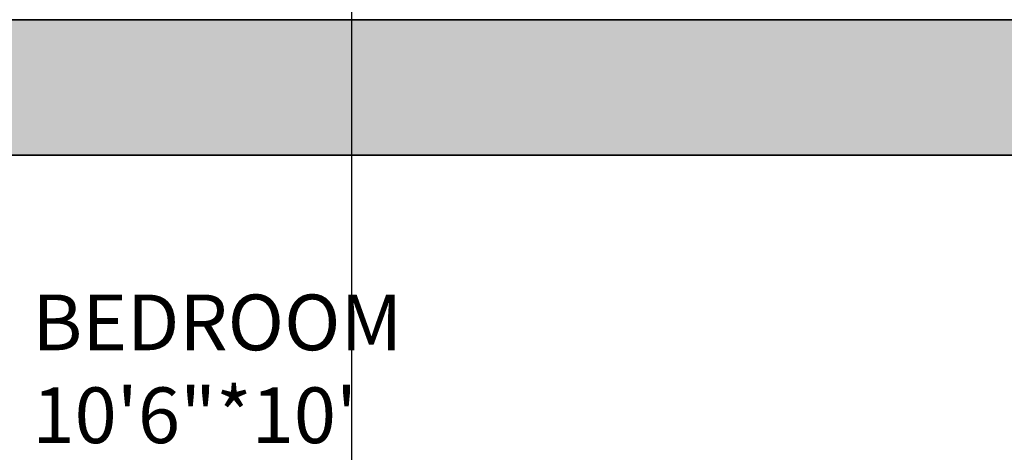
# Model space of a CAD drawing. Units: inches. Extents: x 1998 to 2588, y 1139 to 1977.
# Tile 74 of 134: x 2126 to 2192, y 1860 to 1889. Entities that reach past the tile are written whole.
import ezdxf

# ---------------------------------------------------------------- set-up
doc = ezdxf.new("R2010")
doc.units = ezdxf.units.IN
for name, color, linetype, lineweight in [('A-ANNO-DIMS', 2, 'Continuous', 18), ('A-AREA-IDEN', 7, 'Continuous', 18), ('A-WALL-PATT', 252, 'Continuous', 13), ('WALL', 200, 'Continuous', 35)]:
    doc.layers.add(name, color=color, linetype=linetype, lineweight=lineweight)
doc.styles.get("Standard").update_dxf_attribs({"font": 'arial.ttf'})
doc.dimstyles.get("Standard").update_dxf_attribs({"dimtxt": 0.18, "dimasz": 0.18, "dimexe": 0.18, "dimexo": 0.0625, "dimgap": 0.09, "dimtad": 0, "dimtih": 1, "dimtoh": 1, "dimdec": 4, "dimzin": 0, "dimdsep": 46, "dimtxsty": 'Standard', "dimcen": 0.09, "dimadec": 0, "dimazin": 0, "dimtfac": 1, "dimtdec": 4, "dimtofl": 0, "dimtmove": 0, "dimatfit": 3, "dimfxl": 1, "dimtolj": 1, "dimtzin": 0, "dimarcsym": 0})

# ---------------------------------------------------------------- blocks, each defined once
blk = doc.blocks.new('*D37')
at = {"layer": 'A-ANNO-DIMS', "color": 0, "lineweight": -2, "transparency": 16777216}
for p, q in [((2148.455, 1612.795), (2148.455, 1977.362)), ((2148.635, 1977.182), (2172.73, 1977.182)), ((2197.27, 1977.182), (2173.175, 1977.182)), ((2197.45, 1612.795), (2197.45, 1977.362))]:
    blk.add_line(p, q, dxfattribs=at)
at = {"layer": 'A-ANNO-DIMS', "color": 0, "transparency": 16777216}
for points in [[(2148.635, 1977.212), (2148.635, 1977.152), (2148.455, 1977.182)], [(2197.27, 1977.212), (2197.27, 1977.152), (2197.45, 1977.182)]]:
    blk.add_solid(points, dxfattribs=at)
at = {"layer": 'Defpoints', "color": 0, "transparency": 16777216}
for p in [(2197.45, 1977.182), (2148.455, 1612.732), (2197.45, 1612.732)]:
    blk.add_point(p, dxfattribs=at)
at = {"layer": 'A-ANNO-DIMS', "color": 0, "transparency": 16777216, "insert": (2172.952, 1977.182), "char_height": 0.18, "attachment_point": 5}
blk.add_mtext('\\A1;49', dxfattribs=at)

msp = doc.modelspace()

# ---------------------------------------------------------------- hatches: boundary and pattern name
at = {"layer": 'A-WALL-PATT'}
h = msp.add_hatch(color=256, dxfattribs=at)
h.dxf.hatch_style = 1
h.paths.add_polyline_path([(2222.9729, 1888.7324), (2099.4125, 1888.7324), (2099.4125, 1879.7324), (2222.9729, 1879.7324)])
h.paths.add_polyline_path([(2096.9729, 1868.3278), (2087.9729, 1868.3278), (2087.9729, 1775.637), (2096.9729, 1775.637)])
h.paths.add_polyline_path([(2227.4729, 1868.3278), (2222.9729, 1868.3278), (2222.9729, 1774.3318), (2227.4729, 1774.3318)])
h.paths.add_polyline_path([(2188.3019, 1759.7324), (2138.6074, 1759.7324), (2099.4125, 1759.7324), (2099.4125, 1755.2324), (2176.9729, 1755.2324), (2188.3019, 1755.2324)])
h.paths.add_polyline_path([(2087.9729, 1759.7324), (2059.4729, 1759.7324), (2059.4729, 1702.7324), (2087.9729, 1702.7324), (2087.9729, 1707.2324), (2063.9729, 1707.2324), (2063.9729, 1755.2324), (2087.9729, 1755.2324)])
h.paths.add_polyline_path([(2096.9729, 1755.2324), (2087.9729, 1755.2324), (2087.9729, 1707.2324), (2096.9729, 1707.2324)])
h.paths.add_polyline_path([(2187.0461, 1707.2324), (2105.9729, 1707.2324), (2096.9729, 1707.2324), (2087.9729, 1707.2324), (2087.9729, 1702.7324), (2105.9729, 1702.7324), (2114.9729, 1702.7324), (2187.0461, 1702.7324)])
h.paths.add_polyline_path([(2181.4729, 1719.2028), (2176.9729, 1719.2028), (2176.9729, 1707.2324), (2181.4729, 1707.2324)])
h.paths.add_polyline_path([(2216.0332, 1588.7324), (2114.9729, 1588.7324), (2105.9729, 1588.7324), (2105.9729, 1584.2324), (2216.0332, 1584.2324)])
h.paths.add_polyline_path([(2077.691, 1588.7324), (2061.4729, 1588.7324), (2061.4729, 1584.2324), (2077.691, 1584.2324)])
h.paths.add_polyline_path([(2105.9729, 1588.7324), (2098.0956, 1588.7324), (2098.0956, 1584.2324), (2105.9729, 1584.2324)])
h.paths.add_polyline_path([(2114.9729, 1596.2642), (2110.1012, 1596.2642), (2105.9729, 1596.2642), (2105.9729, 1588.7324), (2114.9729, 1588.7324)])
h.paths.add_polyline_path([(2114.9729, 1584.2324), (2105.9729, 1584.2324), (2105.9729, 1580.249), (2110.1012, 1580.249), (2114.9729, 1580.249)])
h.paths.add_polyline_path([(2114.9729, 1547.7716), (2110.1012, 1547.7716, -0.0318759), (2105.9729, 1548.035), (2105.9729, 1470.2324), (2108.3775, 1470.2324), (2108.3775, 1465.7324), (2186.2943, 1465.7324), (2186.2943, 1470.2324), (2114.9729, 1470.2324)])
h.paths.add_polyline_path([(2227.4729, 1584.2324), (2222.9729, 1584.2324), (2222.9729, 1486.137), (2227.4729, 1486.137)])
h.paths.add_polyline_path([(2295.4138, 1593.2324), (2227.4729, 1593.2324), (2227.4729, 1588.7324), (2295.4138, 1588.7324), (2295.4138, 1591.8729)])
h.paths.add_polyline_path([(2345.9729, 1627.1165), (2341.4729, 1627.1165), (2341.4729, 1593.2324), (2337.2869, 1593.2324), (2337.2869, 1591.8729), (2337.2869, 1588.7324), (2345.9729, 1588.7324)])
h.paths.add_polyline_path([(2291.9729, 1588.7324), (2287.4729, 1588.7324), (2287.4729, 1522.7324), (2291.9729, 1522.7324)])
h.paths.add_polyline_path([(2291.9729, 1522.7324), (2287.4729, 1522.7324), (2227.4729, 1522.7324), (2227.4729, 1518.2324), (2291.9729, 1518.2324)])
h.paths.add_polyline_path([(2295.7347, 1519.5919), (2295.7347, 1522.7324), (2291.9729, 1522.7324), (2291.9729, 1518.2324), (2295.7347, 1518.2324)])
h.paths.add_polyline_path([(2345.9729, 1522.7324), (2337.6078, 1522.7324), (2337.6078, 1519.5919), (2337.6078, 1518.2324), (2341.4729, 1518.2324), (2341.4729, 1488.5616), (2345.9729, 1488.5616)])
h.paths.add_polyline_path([(2345.9729, 1468.1569), (2341.4729, 1468.1569), (2341.4729, 1374.2324), (2227.4729, 1374.2324), (2227.4729, 1369.7324), (2345.9729, 1369.7324)])
h.paths.add_polyline_path([(2345.9729, 1369.7324), (2341.4729, 1369.7324), (2341.4729, 1362.2324), (2345.9729, 1362.2324)])
h.paths.add_polyline_path([(2345.9729, 1317.7324), (2345.9729, 1322.2324), (2341.4729, 1322.2324), (2341.4729, 1285.137), (2345.9729, 1285.137)], flags=17)
h.paths.add_polyline_path([(2356.2096, 1322.2324), (2345.9729, 1322.2324), (2345.9729, 1317.7324), (2356.2096, 1317.7324), (2356.2096, 1319.3088)], flags=17)
h.paths.add_polyline_path([(2393.9729, 1322.2324), (2375.6999, 1322.2324), (2375.6999, 1319.3088, -0.0202458), (2375.636, 1317.7324), (2393.9729, 1317.7324)], flags=17)
h.paths.add_polyline_path([(2398.4729, 1322.2324), (2393.9729, 1322.2324), (2393.9729, 1317.7324), (2393.9729, 1237.7324), (2345.9729, 1237.7324), (2345.9729, 1264.7324), (2341.4729, 1264.7324), (2341.4729, 1228.7324), (2393.9729, 1228.7324), (2482.7412, 1228.7324), (2482.7412, 1237.7324), (2398.4729, 1237.7324), (2398.4729, 1297.1029)])
h.paths.add_polyline_path([(2398.4729, 1362.2324), (2393.9729, 1362.2324), (2393.9729, 1357.7324), (2398.4729, 1357.7324)])
h.paths.add_polyline_path([(2345.9729, 1329.7549), (2341.4729, 1329.7549), (2341.4729, 1322.2324), (2345.9729, 1322.2324)])

# ---------------------------------------------------------------- linework, layer by layer
at = {"layer": 'WALL'}
for p, q in [((2227.4729, 1888.7324), (2087.9729, 1888.7324)), ((2222.9729, 1879.7324), (2099.4125, 1879.7324))]:
    msp.add_line(p, q, dxfattribs=at)

# ---------------------------------------------------------------- texts
at = {"layer": 'A-AREA-IDEN', "insert": (2127.2508, 1870.4864), "char_height": 3.69875, "attachment_point": 1}
msp.add_mtext_dynamic_manual_height_columns('BEDROOM\\P10\'6"*10\'', width=110.572713, gutter_width=18.4938, heights=[0], dxfattribs=at)

# ---------------------------------------------------------------- dimensions: what is measured, and where the dimension line sits
at = {"layer": 'A-ANNO-DIMS'}
dim = msp.add_linear_dim(base=(2197.4499, 1977.1824), p1=(2148.4548, 1612.7324), p2=(2197.4499, 1612.7324), dimstyle='Standard', override={"dimdec": 0, "dimlfac": 1, "dimrnd": 0, "dimzin": 0, "dimdsep": 46, "dimlunit": 2}, dxfattribs=at)
dim.commit()
dim.dimension.update_dxf_attribs({"geometry": '*D37', "text_midpoint": (2172.9524, 1977.1824)})

doc.saveas('drawing.dxf')
